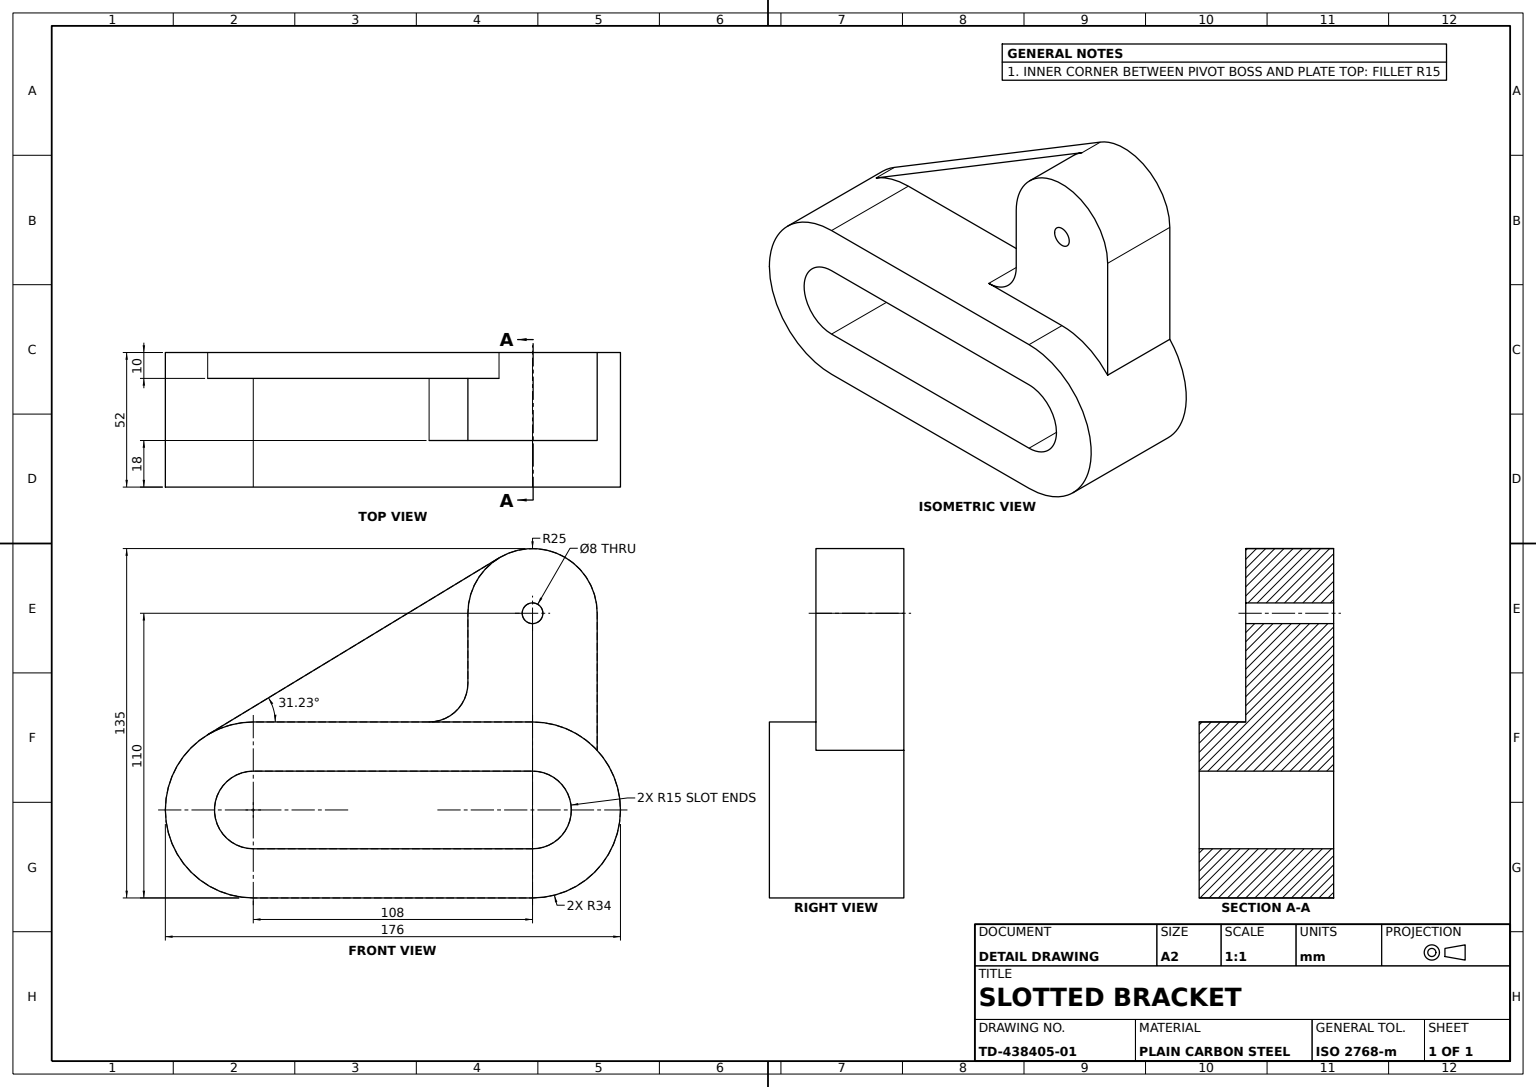
SolidWorks part; units mm, degrees
material "Plain Carbon Steel"
ref_plane "Front Plane" through (0, 0, 0) normal (0, 0, 1) x (1, 0, 0)
ref_plane "Top Plane" through (0, 0, 0) normal (0, 1, 0) x (1, 0, 0)
ref_plane "Right Plane" through (0, 0, 0) normal (1, 0, 0) x (0, 0, -1)
sketch "Link Plate Outline Sketch" plane through (0, 0, 0) normal (0, 0, 1) x (1, 0, 0)
  line L0 (-54, 0) -> (54, 0) construction
  line L2 (-54, 34) -> (54, 34)
  line L3 (-54, -34) -> (54, -34)
  arc A0 (-54, 34) -> (-54, -34) centre (-54, 0) ccw
  arc A1 (54, -34) -> (54, 34) centre (54, 0) ccw
  point P5 (0, 0)
  dimension "D1" = 34
  dimension "D2" = 108
extrude "Link Plate" add sketch "Link Plate Outline Sketch" along normal blind 52
sketch "Link Slot Sketch" plane through (0, 0, 52) normal (0, 0, 1) x (1, 0, 0)
  line L0 (-54, 0) -> (54, 0) construction
  line L2 (-54, 15) -> (54, 15)
  line L3 (-54, -15) -> (54, -15)
  arc A0 (-54, 15) -> (-54, -15) centre (-54, 0) ccw
  arc A1 (54, -15) -> (54, 15) centre (54, 0) ccw
  point P5 (0, 0)
  dimension "D1" = 15
  dimension "D2" = 108
extrude "Link Slot" cut sketch "Link Slot Sketch" against normal blind 52
sketch "Pivot Boss Sketch" plane through (0, 0, 0) normal (0, 0, 1) x (1, 0, 0)
  line L0 (54, 0) -> (54, 76) construction
  line L1 (29, 76) -> (29, 34)
  line L2 (54, 34) -> (-54, 34) construction
  line L3 (79, 76) -> (79, 18.0316)
  line L4 (79, 18.0316) -> (29, 18.0316)
  line L5 (29, 18.0316) -> (29, 34)
  arc A0 (79, 76) -> (29, 76) centre (54, 76) ccw
  dimension "D1" = 25
  dimension "D2" = 15.9684
  dimension "D3" = 57.9684
extrude "Pivot Boss" add sketch "Pivot Boss Sketch" along normal blind 34
sketch "Pivot Pin Hole Sketch" plane through (0, 0, 34) normal (0, 0, 1) x (1, 0, 0)
  circle A0 centre (54, 76) radius 4
  dimension "D1" = 8
extrude "Pivot Pin Hole" cut sketch "Pivot Pin Hole Sketch" against normal blind 34
sketch "Support Rib Sketch" plane through (0, 0, 0) normal (0, 0, 1) x (1, 0, 0)
  line L0 (-71.6263, 29.0743) -> (41.0395, 97.3781)
  arc A1 (-54, 34) -> (-54, -34) centre (-54, 0) ccw construction
  arc A2 (79, 76) -> (29, 76) centre (54, 76) ccw construction
  dimension "D1" = 112.6658
  dimension "D2" = 68.3039
rib "Support Rib 10mm" sketch "Support Rib Sketch" sketch "Support Rib Sketch" thickness 10 parameters "D1"=10
fillet "Edge Fillets R15" radius 15 1 edges at (29, 34, 22)
